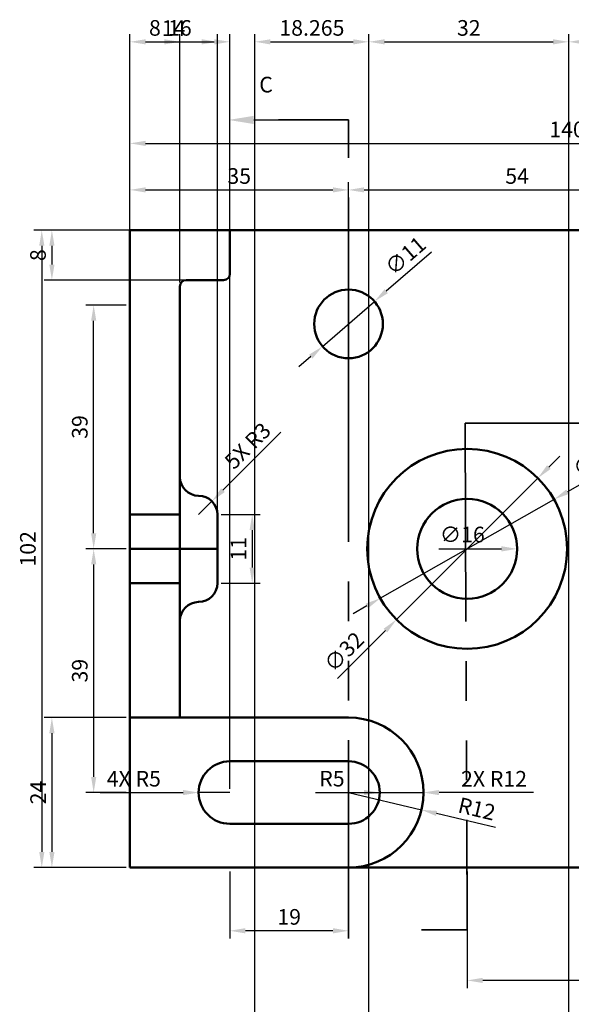
# Model space of a CAD drawing. Units: millimetres. Extents: x 2432 to 2611, y 2100 to 2357.
# Tile 2 of 3: x 2432 to 2521, y 2199 to 2357. Entities that reach past the tile are written whole.
import ezdxf
from ezdxf import colors
from ezdxf.entities.mleader import LeaderData, LeaderLine
from ezdxf.math import Vec2, Vec3

# ---------------------------------------------------------------- set-up
doc = ezdxf.new("R2010")
doc.units = ezdxf.units.MM
doc.linetypes.add('PHANTOM', pattern=[63.5, 31.75, -6.35, 6.35, -6.35, 6.35, -6.35])
for name, color, linetype, lineweight in [('M-DIMS', 2, 'Continuous', 25), ('M-OUTL', 7, 'Continuous', 50), ('M-SECT', 1, 'PHANTOM', 35), ('M-TEXT', 3, 'Continuous', 25)]:
    doc.layers.add(name, color=color, linetype=linetype, lineweight=lineweight)
doc.styles.get("Standard").update_dxf_attribs({"font": 'arial.ttf'})
doc.dimstyles.new('ISO-25', dxfattribs={"dimtxt": 2.5, "dimasz": 2.5, "dimexe": 1.25, "dimexo": 0.625, "dimtad": 1, "dimtxsty": 'Standard', "dimcen": 2.5, "dimadec": 0, "dimazin": 0, "dimtfac": 1, "dimtmove": 0, "dimatfit": 3, "dimfxl": 1, "dimarcsym": 0})

# ---------------------------------------------------------------- blocks, each defined once
blk = doc.blocks.new('*D1')
at = {"layer": 'Defpoints', "color": 0, "transparency": 16777216}
for p in [(2485.07, 2329.49), (2450.07, 2323.05), (2485.07, 2323.05)]:
    blk.add_point(p, dxfattribs=at)
at = {"layer": 'M-DIMS', "color": 0, "lineweight": -2, "transparency": 16777216}
for p, q in [((2450.07, 2323.67), (2450.07, 2330.74)), ((2485.07, 2323.67), (2485.07, 2330.74)), ((2452.57, 2329.49), (2482.57, 2329.49))]:
    blk.add_line(p, q, dxfattribs=at)
at = {"layer": 'M-DIMS', "color": 0, "transparency": 16777216}
for points in [[(2452.57, 2329.91), (2452.57, 2329.08), (2450.07, 2329.49)], [(2482.57, 2329.91), (2482.57, 2329.08), (2485.07, 2329.49)]]:
    blk.add_solid(points, dxfattribs=at)
at = {"layer": 'M-DIMS', "color": 0, "transparency": 16777216, "insert": (2467.57, 2331.39), "char_height": 2.5, "attachment_point": 5}
blk.add_mtext('35', dxfattribs=at)
blk = doc.blocks.new('*D2')
at = {"layer": 'Defpoints', "color": 0, "transparency": 16777216}
for p in [(2539.07, 2329.49), (2485.07, 2323.05), (2539.07, 2323.05)]:
    blk.add_point(p, dxfattribs=at)
at = {"layer": 'M-DIMS', "color": 0, "lineweight": -2, "transparency": 16777216}
for p, q in [((2485.07, 2323.67), (2485.07, 2330.74)), ((2539.07, 2323.67), (2539.07, 2330.74)), ((2487.57, 2329.49), (2536.57, 2329.49))]:
    blk.add_line(p, q, dxfattribs=at)
at = {"layer": 'M-DIMS', "color": 0, "transparency": 16777216}
for points in [[(2487.57, 2329.91), (2487.57, 2329.08), (2485.07, 2329.49)], [(2536.57, 2329.91), (2536.57, 2329.08), (2539.07, 2329.49)]]:
    blk.add_solid(points, dxfattribs=at)
at = {"layer": 'M-DIMS', "color": 0, "transparency": 16777216, "insert": (2512.07, 2331.39), "char_height": 2.5, "attachment_point": 5}
blk.add_mtext('54', dxfattribs=at)
blk = doc.blocks.new('*D3')
at = {"layer": 'Defpoints', "color": 0, "transparency": 16777216}
for p in [(2590.07, 2336.94), (2450.07, 2323.05), (2590.07, 2323.05)]:
    blk.add_point(p, dxfattribs=at)
at = {"layer": 'M-DIMS', "color": 0, "lineweight": -2, "transparency": 16777216}
for p, q in [((2450.07, 2323.67), (2450.07, 2338.19)), ((2452.57, 2336.94), (2587.57, 2336.94)), ((2590.07, 2323.67), (2590.07, 2338.19))]:
    blk.add_line(p, q, dxfattribs=at)
at = {"layer": 'M-DIMS', "color": 0, "transparency": 16777216}
for points in [[(2452.57, 2337.35), (2452.57, 2336.52), (2450.07, 2336.94)], [(2587.57, 2337.35), (2587.57, 2336.52), (2590.07, 2336.94)]]:
    blk.add_solid(points, dxfattribs=at)
at = {"layer": 'M-DIMS', "color": 0, "transparency": 16777216, "insert": (2520.07, 2338.84), "char_height": 2.5, "attachment_point": 5}
blk.add_mtext('140', dxfattribs=at)
blk = doc.blocks.new('*D9')
at = {"layer": 'Defpoints', "color": 0, "transparency": 16777216}
for p in [(2504.07, 2221.05), (2590.07, 2221.05), (2504.07, 2202.99)]:
    blk.add_point(p, dxfattribs=at)
at = {"layer": 'M-DIMS', "color": 0, "lineweight": -2, "transparency": 16777216}
for p, q in [((2504.07, 2220.42), (2504.07, 2201.74)), ((2590.07, 2220.42), (2590.07, 2201.74)), ((2587.57, 2202.99), (2506.57, 2202.99))]:
    blk.add_line(p, q, dxfattribs=at)
at = {"layer": 'M-DIMS', "color": 0, "transparency": 16777216}
for points in [[(2506.57, 2203.4), (2506.57, 2202.57), (2504.07, 2202.99)], [(2587.57, 2203.4), (2587.57, 2202.57), (2590.07, 2202.99)]]:
    blk.add_solid(points, dxfattribs=at)
at = {"layer": 'M-DIMS', "color": 0, "transparency": 16777216, "insert": (2547.07, 2204.89), "char_height": 2.5, "attachment_point": 5}
blk.add_mtext('86', dxfattribs=at)
blk = doc.blocks.new('*D10')
at = {"layer": 'Defpoints', "color": 0, "transparency": 16777216}
for p in [(2466.07, 2221.05), (2485.07, 2221.05), (2466.07, 2210.93)]:
    blk.add_point(p, dxfattribs=at)
at = {"layer": 'M-DIMS', "color": 0, "lineweight": -2, "transparency": 16777216}
for p, q in [((2466.07, 2220.42), (2466.07, 2209.68)), ((2485.07, 2220.42), (2485.07, 2209.68)), ((2482.57, 2210.93), (2468.57, 2210.93))]:
    blk.add_line(p, q, dxfattribs=at)
at = {"layer": 'M-DIMS', "color": 0, "transparency": 16777216}
for points in [[(2468.57, 2211.35), (2468.57, 2210.51), (2466.07, 2210.93)], [(2482.57, 2211.35), (2482.57, 2210.51), (2485.07, 2210.93)]]:
    blk.add_solid(points, dxfattribs=at)
at = {"layer": 'M-DIMS', "color": 0, "transparency": 16777216, "insert": (2475.57, 2212.83), "char_height": 2.5, "attachment_point": 5}
blk.add_mtext('19', dxfattribs=at)
blk = doc.blocks.new('*D11')
at = {"layer": 'Defpoints', "color": 0, "transparency": 16777216}
for p in [(2464.07, 2277.55), (2464.07, 2266.55), (2469.65, 2266.55)]:
    blk.add_point(p, dxfattribs=at)
at = {"layer": 'M-DIMS', "color": 0, "lineweight": -2, "transparency": 16777216}
for p, q in [((2464.7, 2277.55), (2470.9, 2277.55)), ((2469.65, 2275.05), (2469.65, 2269.05)), ((2464.7, 2266.55), (2470.9, 2266.55))]:
    blk.add_line(p, q, dxfattribs=at)
at = {"layer": 'M-DIMS', "color": 0, "transparency": 16777216}
for points in [[(2469.23, 2275.05), (2470.06, 2275.05), (2469.65, 2277.55)], [(2469.23, 2269.05), (2470.06, 2269.05), (2469.65, 2266.55)]]:
    blk.add_solid(points, dxfattribs=at)
at = {"layer": 'M-DIMS', "color": 0, "transparency": 16777216, "insert": (2467.77, 2272.05), "char_height": 2.5, "attachment_point": 5, "rotation": 90}
blk.add_mtext('11', dxfattribs=at)
blk = doc.blocks.new('*D12')
at = {"layer": 'Defpoints', "color": 0, "transparency": 16777216}
for p in [(2444.26, 2311.05), (2450.07, 2311.05), (2450.07, 2272.05)]:
    blk.add_point(p, dxfattribs=at)
at = {"layer": 'M-DIMS', "color": 0, "lineweight": -2, "transparency": 16777216}
for p, q in [((2449.45, 2311.05), (2443.01, 2311.05)), ((2444.26, 2274.55), (2444.26, 2308.55)), ((2449.45, 2272.05), (2443.01, 2272.05))]:
    blk.add_line(p, q, dxfattribs=at)
at = {"layer": 'M-DIMS', "color": 0, "transparency": 16777216}
for points in [[(2443.85, 2308.55), (2444.68, 2308.55), (2444.26, 2311.05)], [(2443.85, 2274.55), (2444.68, 2274.55), (2444.26, 2272.05)]]:
    blk.add_solid(points, dxfattribs=at)
at = {"layer": 'M-DIMS', "color": 0, "transparency": 16777216, "insert": (2442.36, 2291.55), "char_height": 2.5, "attachment_point": 5, "rotation": 90}
blk.add_mtext('39', dxfattribs=at)
blk = doc.blocks.new('*D13')
at = {"layer": 'Defpoints', "color": 0, "transparency": 16777216}
for p in [(2450.07, 2272.05), (2444.26, 2233.05), (2450.07, 2233.05)]:
    blk.add_point(p, dxfattribs=at)
at = {"layer": 'M-DIMS', "color": 0, "lineweight": -2, "transparency": 16777216}
for p, q in [((2449.45, 2272.05), (2443.01, 2272.05)), ((2444.26, 2269.55), (2444.26, 2235.55)), ((2449.45, 2233.05), (2443.01, 2233.05))]:
    blk.add_line(p, q, dxfattribs=at)
at = {"layer": 'M-DIMS', "color": 0, "transparency": 16777216}
for points in [[(2443.85, 2269.55), (2444.68, 2269.55), (2444.26, 2272.05)], [(2443.85, 2235.55), (2444.68, 2235.55), (2444.26, 2233.05)]]:
    blk.add_solid(points, dxfattribs=at)
at = {"layer": 'M-DIMS', "color": 0, "transparency": 16777216, "insert": (2442.36, 2252.55), "char_height": 2.5, "attachment_point": 5, "rotation": 90}
blk.add_mtext('39', dxfattribs=at)
blk = doc.blocks.new('*D14')
at = {"layer": 'Defpoints', "color": 0, "transparency": 16777216}
for p in [(2450.07, 2323.05), (2435.95, 2221.05), (2450.07, 2221.05)]:
    blk.add_point(p, dxfattribs=at)
at = {"layer": 'M-DIMS', "color": 0, "lineweight": -2, "transparency": 16777216}
for p, q in [((2449.45, 2323.05), (2434.7, 2323.05)), ((2435.95, 2320.55), (2435.95, 2223.55)), ((2449.45, 2221.05), (2434.7, 2221.05))]:
    blk.add_line(p, q, dxfattribs=at)
at = {"layer": 'M-DIMS', "color": 0, "transparency": 16777216}
for points in [[(2435.54, 2320.55), (2436.37, 2320.55), (2435.95, 2323.05)], [(2435.54, 2223.55), (2436.37, 2223.55), (2435.95, 2221.05)]]:
    blk.add_solid(points, dxfattribs=at)
at = {"layer": 'M-DIMS', "color": 0, "transparency": 16777216, "insert": (2434.05, 2272.05), "char_height": 2.5, "attachment_point": 5, "rotation": 90}
blk.add_mtext('102', dxfattribs=at)
blk = doc.blocks.new('*D15')
at = {"layer": 'Defpoints', "color": 0, "transparency": 16777216}
for p in [(2489.24, 2311.65), (2480.91, 2304.45)]:
    blk.add_point(p, dxfattribs=at)
at = {"layer": 'M-DIMS', "color": 0, "lineweight": -2, "transparency": 16777216}
for p, q in [((2498.36, 2319.54), (2491.13, 2313.28)), ((2480.91, 2304.45), (2489.24, 2311.65)), ((2479.02, 2302.82), (2477.13, 2301.18))]:
    blk.add_line(p, q, dxfattribs=at)
at = {"layer": 'M-DIMS', "color": 0, "transparency": 16777216}
for points in [[(2490.85, 2313.6), (2491.4, 2312.97), (2489.24, 2311.65)], [(2478.75, 2303.13), (2479.3, 2302.5), (2480.91, 2304.45)]]:
    blk.add_solid(points, dxfattribs=at)
at = {"layer": 'M-DIMS', "color": 0, "transparency": 16777216, "insert": (2494.4, 2318.72), "char_height": 2.5, "attachment_point": 5, "rotation": 40.8461}
blk.add_mtext('∅11', dxfattribs=at)
blk = doc.blocks.new('*D19')
at = {"layer": 'Defpoints', "color": 0, "transparency": 16777216}
for p in [(2496.07, 2272.05), (2512.07, 2272.05)]:
    blk.add_point(p, dxfattribs=at)
at = {"layer": 'M-DIMS', "color": 0, "lineweight": -2, "transparency": 16777216}
blk.add_line((2499.53, 2272.05), (2509.57, 2272.05), dxfattribs=at)
at = {"layer": 'M-DIMS', "color": 0, "transparency": 16777216}
blk.add_solid([(2509.57, 2272.47), (2509.57, 2271.63), (2512.07, 2272.05)], dxfattribs=at)
at = {"layer": 'M-DIMS', "color": 0, "transparency": 16777216, "insert": (2503.3, 2274.02), "char_height": 2.5, "attachment_point": 5}
blk.add_mtext('∅16', dxfattribs=at)
blk = doc.blocks.new('*D20')
at = {"layer": 'Defpoints', "color": 0, "transparency": 16777216}
for p in [(2517.98, 2279.96), (2490.16, 2264.14)]:
    blk.add_point(p, dxfattribs=at)
at = {"layer": 'M-DIMS', "color": 0, "lineweight": -2, "transparency": 16777216}
for p, q in [((2528.87, 2286.15), (2520.16, 2281.19)), ((2490.16, 2264.14), (2517.98, 2279.96)), ((2487.99, 2262.91), (2485.82, 2261.67))]:
    blk.add_line(p, q, dxfattribs=at)
at = {"layer": 'M-DIMS', "color": 0, "transparency": 16777216}
for points in [[(2519.95, 2281.55), (2520.36, 2280.83), (2517.98, 2279.96)], [(2487.79, 2263.27), (2488.2, 2262.54), (2490.16, 2264.14)]]:
    blk.add_solid(points, dxfattribs=at)
at = {"layer": 'M-DIMS', "color": 0, "transparency": 16777216, "insert": (2524.63, 2286), "char_height": 2.5, "attachment_point": 5, "rotation": 29.6157}
blk.add_mtext('∅32', dxfattribs=at)
blk = doc.blocks.new('*D21')
at = {"layer": 'Defpoints', "color": 0, "transparency": 16777216}
for p in [(2485.07, 2233.05), (2490.07, 2233.05)]:
    blk.add_point(p, dxfattribs=at)
at = {"layer": 'M-DIMS', "color": 0, "lineweight": -2, "transparency": 16777216}
blk.add_line((2479.77, 2233.05), (2487.57, 2233.05), dxfattribs=at)
at = {"layer": 'M-DIMS', "color": 0, "transparency": 16777216}
blk.add_solid([(2487.57, 2233.47), (2487.57, 2232.63), (2490.07, 2233.05)], dxfattribs=at)
at = {"layer": 'M-DIMS', "color": 0, "transparency": 16777216, "insert": (2482.42, 2234.95), "char_height": 2.5, "attachment_point": 5}
blk.add_mtext('R5', dxfattribs=at)
blk = doc.blocks.new('*D22')
at = {"layer": 'Defpoints', "color": 0, "transparency": 16777216}
for p in [(2485.07, 2233.05), (2496.75, 2230.28)]:
    blk.add_point(p, dxfattribs=at)
at = {"layer": 'M-DIMS', "color": 0, "lineweight": -2, "transparency": 16777216}
for p, q in [((2485.07, 2233.05), (2496.75, 2230.28)), ((2508.62, 2227.47), (2499.18, 2229.7))]:
    blk.add_line(p, q, dxfattribs=at)
at = {"layer": 'M-DIMS', "color": 0, "transparency": 16777216}
blk.add_solid([(2499.28, 2230.11), (2499.09, 2229.3), (2496.75, 2230.28)], dxfattribs=at)
at = {"layer": 'M-DIMS', "color": 0, "transparency": 16777216, "insert": (2505.55, 2230.13), "char_height": 2.5, "attachment_point": 5, "rotation": 346.6592}
blk.add_mtext('R12', dxfattribs=at)
blk = doc.blocks.new('*D34')
at = {"layer": 'Defpoints', "color": 0, "transparency": 16777216}
for p in [(2458.07, 2353.19), (2450.07, 2323.05), (2458.07, 2314.05)]:
    blk.add_point(p, dxfattribs=at)
at = {"layer": 'M-DIMS', "color": 0, "lineweight": -2, "transparency": 16777216}
for p, q in [((2450.07, 2323.67), (2450.07, 2354.44)), ((2458.07, 2314.67), (2458.07, 2354.44)), ((2452.57, 2353.19), (2455.57, 2353.19))]:
    blk.add_line(p, q, dxfattribs=at)
at = {"layer": 'M-DIMS', "color": 0, "transparency": 16777216}
for points in [[(2452.57, 2353.6), (2452.57, 2352.77), (2450.07, 2353.19)], [(2455.57, 2353.6), (2455.57, 2352.77), (2458.07, 2353.19)]]:
    blk.add_solid(points, dxfattribs=at)
at = {"layer": 'M-DIMS', "color": 0, "transparency": 16777216, "insert": (2454.07, 2355.09), "char_height": 2.5, "attachment_point": 5}
blk.add_mtext('8', dxfattribs=at)
blk = doc.blocks.new('*D35')
at = {"layer": 'Defpoints', "color": 0, "transparency": 16777216}
for p in [(2466.07, 2353.19), (2450.07, 2323.05), (2466.07, 2323.05)]:
    blk.add_point(p, dxfattribs=at)
at = {"layer": 'M-DIMS', "color": 0, "lineweight": -2, "transparency": 16777216}
for p, q in [((2450.07, 2323.67), (2450.07, 2354.44)), ((2466.07, 2323.67), (2466.07, 2354.44)), ((2452.57, 2353.19), (2463.57, 2353.19))]:
    blk.add_line(p, q, dxfattribs=at)
at = {"layer": 'M-DIMS', "color": 0, "transparency": 16777216}
for points in [[(2452.57, 2353.6), (2452.57, 2352.77), (2450.07, 2353.19)], [(2463.57, 2353.6), (2463.57, 2352.77), (2466.07, 2353.19)]]:
    blk.add_solid(points, dxfattribs=at)
at = {"layer": 'M-DIMS', "color": 0, "transparency": 16777216, "insert": (2458.07, 2355.09), "char_height": 2.5, "attachment_point": 5}
blk.add_mtext('16', dxfattribs=at)
blk = doc.blocks.new('*D36')
at = {"layer": 'Defpoints', "color": 0, "transparency": 16777216}
for p in [(2466.07, 2323.05), (2437.57, 2315.05), (2462.67, 2315.05)]:
    blk.add_point(p, dxfattribs=at)
at = {"layer": 'M-DIMS', "color": 0, "lineweight": -2, "transparency": 16777216}
for p, q in [((2465.45, 2323.05), (2436.32, 2323.05)), ((2437.57, 2320.55), (2437.57, 2317.55)), ((2462.05, 2315.05), (2436.32, 2315.05))]:
    blk.add_line(p, q, dxfattribs=at)
at = {"layer": 'M-DIMS', "color": 0, "transparency": 16777216}
for points in [[(2437.16, 2320.55), (2437.99, 2320.55), (2437.57, 2323.05)], [(2437.16, 2317.55), (2437.99, 2317.55), (2437.57, 2315.05)]]:
    blk.add_solid(points, dxfattribs=at)
at = {"layer": 'M-DIMS', "color": 0, "transparency": 16777216, "insert": (2435.67, 2319.05), "char_height": 2.5, "attachment_point": 5, "rotation": 90}
blk.add_mtext('8', dxfattribs=at)
blk = doc.blocks.new('*D40')
at = {"layer": 'Defpoints', "color": 0, "transparency": 16777216}
for p in [(2450.07, 2245.05), (2437.57, 2221.05), (2450.07, 2221.05)]:
    blk.add_point(p, dxfattribs=at)
at = {"layer": 'M-DIMS', "color": 0, "lineweight": -2, "transparency": 16777216}
for p, q in [((2449.45, 2245.05), (2436.32, 2245.05)), ((2437.57, 2242.55), (2437.57, 2223.55)), ((2449.45, 2221.05), (2436.32, 2221.05))]:
    blk.add_line(p, q, dxfattribs=at)
at = {"layer": 'M-DIMS', "color": 0, "transparency": 16777216}
for points in [[(2437.16, 2242.55), (2437.99, 2242.55), (2437.57, 2245.05)], [(2437.16, 2223.55), (2437.99, 2223.55), (2437.57, 2221.05)]]:
    blk.add_solid(points, dxfattribs=at)
at = {"layer": 'M-DIMS', "color": 0, "transparency": 16777216, "insert": (2435.69, 2233.05), "char_height": 2.5, "attachment_point": 5, "rotation": 90}
blk.add_mtext('24', dxfattribs=at)
blk = doc.blocks.new('*D41')
at = {"layer": 'Defpoints', "color": 0, "transparency": 16777216}
for p in [(2466.07, 2353.19), (2466.07, 2233.05), (2450.07, 2221.05)]:
    blk.add_point(p, dxfattribs=at)
at = {"layer": 'M-DIMS', "color": 0, "lineweight": -2, "transparency": 16777216}
for p, q in [((2450.07, 2221.67), (2450.07, 2354.44)), ((2466.07, 2233.67), (2466.07, 2354.44)), ((2452.57, 2353.19), (2463.57, 2353.19))]:
    blk.add_line(p, q, dxfattribs=at)
at = {"layer": 'M-DIMS', "color": 0, "transparency": 16777216}
for points in [[(2452.57, 2353.6), (2452.57, 2352.77), (2450.07, 2353.19)], [(2463.57, 2353.6), (2463.57, 2352.77), (2466.07, 2353.19)]]:
    blk.add_solid(points, dxfattribs=at)
at = {"layer": 'M-DIMS', "color": 0, "transparency": 16777216, "insert": (2458.07, 2355.09), "char_height": 2.5, "attachment_point": 5}
blk.add_mtext('16', dxfattribs=at)
blk = doc.blocks.new('*D42')
at = {"layer": 'Defpoints', "color": 0, "transparency": 16777216}
for p in [(2464.07, 2353.19), (2450.07, 2277.55), (2464.07, 2272.05)]:
    blk.add_point(p, dxfattribs=at)
at = {"layer": 'M-DIMS', "color": 0, "lineweight": -2, "transparency": 16777216}
for p, q in [((2450.07, 2278.17), (2450.07, 2354.44)), ((2464.07, 2272.67), (2464.07, 2354.44)), ((2452.57, 2353.19), (2461.57, 2353.19))]:
    blk.add_line(p, q, dxfattribs=at)
at = {"layer": 'M-DIMS', "color": 0, "transparency": 16777216}
for points in [[(2452.57, 2353.6), (2452.57, 2352.77), (2450.07, 2353.19)], [(2461.57, 2353.6), (2461.57, 2352.77), (2464.07, 2353.19)]]:
    blk.add_solid(points, dxfattribs=at)
at = {"layer": 'M-DIMS', "color": 0, "transparency": 16777216, "insert": (2457.07, 2355.07), "char_height": 2.5, "attachment_point": 5}
blk.add_mtext('14', dxfattribs=at)
blk = doc.blocks.new('*D43')
at = {"layer": 'Defpoints', "color": 0, "transparency": 16777216}
for p in [(2488.34, 2353.19), (2470.07, 2151.26), (2488.34, 2145.26)]:
    blk.add_point(p, dxfattribs=at)
at = {"layer": 'M-DIMS', "color": 0, "lineweight": -2, "transparency": 16777216}
for p, q in [((2470.07, 2151.89), (2470.07, 2354.44)), ((2488.34, 2145.89), (2488.34, 2354.44)), ((2472.57, 2353.19), (2485.84, 2353.19))]:
    blk.add_line(p, q, dxfattribs=at)
at = {"layer": 'M-DIMS', "color": 0, "transparency": 16777216}
for points in [[(2472.57, 2353.6), (2472.57, 2352.77), (2470.07, 2353.19)], [(2485.84, 2353.6), (2485.84, 2352.77), (2488.34, 2353.19)]]:
    blk.add_solid(points, dxfattribs=at)
at = {"layer": 'M-DIMS', "color": 0, "transparency": 16777216, "insert": (2479.21, 2355.09), "char_height": 2.5, "attachment_point": 5}
blk.add_mtext('18.265', dxfattribs=at)
blk = doc.blocks.new('*D44')
at = {"layer": 'Defpoints', "color": 0, "transparency": 16777216}
for p in [(2520.34, 2353.19), (2488.34, 2145.26), (2520.34, 2145.26)]:
    blk.add_point(p, dxfattribs=at)
at = {"layer": 'M-DIMS', "color": 0, "lineweight": -2, "transparency": 16777216}
for p, q in [((2488.34, 2145.89), (2488.34, 2354.44)), ((2520.34, 2145.89), (2520.34, 2354.44)), ((2490.84, 2353.19), (2517.84, 2353.19))]:
    blk.add_line(p, q, dxfattribs=at)
at = {"layer": 'M-DIMS', "color": 0, "transparency": 16777216}
for points in [[(2490.84, 2353.6), (2490.84, 2352.77), (2488.34, 2353.19)], [(2517.84, 2353.6), (2517.84, 2352.77), (2520.34, 2353.19)]]:
    blk.add_solid(points, dxfattribs=at)
at = {"layer": 'M-DIMS', "color": 0, "transparency": 16777216, "insert": (2504.34, 2355.09), "char_height": 2.5, "attachment_point": 5}
blk.add_mtext('32', dxfattribs=at)
blk = doc.blocks.new('*D45')
at = {"layer": 'Defpoints', "color": 0, "transparency": 16777216}
for p in [(2534.07, 2353.19), (2534.07, 2151.26), (2520.34, 2145.26)]:
    blk.add_point(p, dxfattribs=at)
at = {"layer": 'M-DIMS', "color": 0, "lineweight": -2, "transparency": 16777216}
for p, q in [((2520.34, 2145.89), (2520.34, 2354.44)), ((2534.07, 2151.89), (2534.07, 2354.44)), ((2522.84, 2353.19), (2531.57, 2353.19))]:
    blk.add_line(p, q, dxfattribs=at)
at = {"layer": 'M-DIMS', "color": 0, "transparency": 16777216}
for points in [[(2522.84, 2353.6), (2522.84, 2352.77), (2520.34, 2353.19)], [(2531.57, 2353.6), (2531.57, 2352.77), (2534.07, 2353.19)]]:
    blk.add_solid(points, dxfattribs=at)
at = {"layer": 'M-DIMS', "color": 0, "transparency": 16777216, "insert": (2527.21, 2355.09), "char_height": 2.5, "attachment_point": 5}
blk.add_mtext('13.735', dxfattribs=at)
blk = doc.blocks.new('*D51')
at = {"layer": 'Defpoints', "color": 0, "transparency": 16777216}
for p in [(2515.39, 2283.36), (2492.76, 2260.74)]:
    blk.add_point(p, dxfattribs=at)
at = {"layer": 'M-DIMS', "color": 0, "lineweight": -2, "transparency": 16777216}
for p, q in [((2517.16, 2285.13), (2518.93, 2286.9)), ((2515.39, 2283.36), (2492.76, 2260.74)), ((2483.31, 2251.29), (2490.99, 2258.97))]:
    blk.add_line(p, q, dxfattribs=at)
at = {"layer": 'M-DIMS', "color": 0, "transparency": 16777216}
for points in [[(2516.86, 2285.42), (2517.45, 2284.83), (2515.39, 2283.36)], [(2490.7, 2259.27), (2491.28, 2258.68), (2492.76, 2260.74)]]:
    blk.add_solid(points, dxfattribs=at)
at = {"layer": 'M-DIMS', "color": 0, "transparency": 16777216, "insert": (2484.57, 2255.35), "char_height": 2.5, "attachment_point": 5, "rotation": 44.9868}
blk.add_mtext('∅32', dxfattribs=at)
blk = doc.blocks.new('*D52')
at = {"layer": 'Defpoints', "color": 0, "transparency": 16777216}
for p in [(2485.07, 2233.05), (2497.07, 2233.05)]:
    blk.add_point(p, dxfattribs=at)
at = {"layer": 'M-DIMS', "color": 0, "lineweight": -2, "transparency": 16777216}
for p, q in [((2485.07, 2233.05), (2497.07, 2233.05)), ((2514.69, 2233.05), (2499.57, 2233.05))]:
    blk.add_line(p, q, dxfattribs=at)
at = {"layer": 'M-DIMS', "color": 0, "transparency": 16777216}
blk.add_solid([(2499.57, 2233.47), (2499.57, 2232.63), (2497.07, 2233.05)], dxfattribs=at)
at = {"layer": 'M-DIMS', "color": 0, "transparency": 16777216, "insert": (2508.38, 2234.93), "char_height": 2.5, "attachment_point": 5, "rotation": 359.9985}
blk.add_mtext('2X R12', dxfattribs=at)
blk = doc.blocks.new('*D53')
at = {"layer": 'Defpoints', "color": 0, "transparency": 16777216}
for p in [(2461.07, 2233.05), (2466.07, 2233.05)]:
    blk.add_point(p, dxfattribs=at)
at = {"layer": 'M-DIMS', "color": 0, "lineweight": -2, "transparency": 16777216}
for p, q in [((2445.3, 2233.05), (2458.57, 2233.05)), ((2466.07, 2233.05), (2461.07, 2233.05))]:
    blk.add_line(p, q, dxfattribs=at)
at = {"layer": 'M-DIMS', "color": 0, "transparency": 16777216}
blk.add_solid([(2458.57, 2233.47), (2458.57, 2232.63), (2461.07, 2233.05)], dxfattribs=at)
at = {"layer": 'M-DIMS', "color": 0, "transparency": 16777216, "insert": (2450.69, 2234.94), "char_height": 2.5, "attachment_point": 5, "rotation": 0.0036}
blk.add_mtext('4X R5', dxfattribs=at)
blk = doc.blocks.new('*D55')
at = {"layer": 'Defpoints', "color": 0, "transparency": 16777216}
for p in [(2463.2, 2279.67), (2461.07, 2277.55)]:
    blk.add_point(p, dxfattribs=at)
at = {"layer": 'M-DIMS', "color": 0, "lineweight": -2, "transparency": 16777216}
for p, q in [((2474.26, 2290.74), (2464.96, 2281.44)), ((2461.07, 2277.55), (2463.2, 2279.67))]:
    blk.add_line(p, q, dxfattribs=at)
at = {"layer": 'M-DIMS', "color": 0, "transparency": 16777216}
blk.add_solid([(2464.67, 2281.73), (2465.26, 2281.14), (2463.2, 2279.67)], dxfattribs=at)
at = {"layer": 'M-DIMS', "color": 0, "transparency": 16777216, "insert": (2469.15, 2288.32), "char_height": 2.5, "attachment_point": 5, "rotation": 45.0031}
blk.add_mtext('5X R3', dxfattribs=at)

msp = doc.modelspace()

# ---------------------------------------------------------------- linework, layer by layer
at = {"layer": 'M-OUTL'}
for p, q in [((2450.0745, 2323.0493), (2590.0745, 2323.0493)), ((2450.0745, 2221.0493), (2450.0745, 2323.0493)), ((2450.0745, 2323.0493), (2485.0745, 2323.0493)), ((2485.0745, 2323.0493), (2466.0745, 2323.0493)), ((2466.0745, 2316.0493), (2466.0745, 2323.0493)), ((2459.2745, 2315.0493), (2459.0745, 2315.0493)), ((2462.6745, 2315.0493), (2459.2745, 2315.0493)), ((2465.0745, 2315.0493), (2462.6745, 2315.0493)), ((2458.0745, 2314.0493), (2458.0745, 2245.0493)), ((2458.0745, 2277.5493), (2458.0745, 2280.5493)), ((2458.0745, 2277.5493), (2450.0745, 2277.5493)), ((2464.0745, 2272.0493), (2464.0745, 2277.5493)), ((2464.0745, 2277.5493), (2464.0745, 2272.0493)), ((2450.0745, 2272.0493), (2464.0745, 2272.0493)), ((2464.0745, 2272.0493), (2464.0745, 2266.5493)), ((2458.0745, 2266.5493), (2450.0745, 2266.5493)), ((2458.0745, 2266.5493), (2458.0745, 2263.5493)), ((2485.0745, 2245.0493), (2450.0745, 2245.0493)), ((2466.0745, 2238.0493), (2485.0745, 2238.0493)), ((2466.0745, 2228.0493), (2485.0745, 2228.0493)), ((2590.0745, 2221.0493), (2450.0745, 2221.0493))]:
    msp.add_line(p, q, dxfattribs=at)
for centre, radius in [((2485.0745, 2308.0493), 5.5), ((2504.0745, 2272.0493), 16), ((2504.0745, 2272.0493), 8)]:
    msp.add_circle(centre, radius, dxfattribs=at)
for centre, radius, start, end in [((2459.0745, 2314.0493), 1, 90, 180), ((2465.0745, 2316.0493), 1, 270, 0), ((2461.0745, 2283.5493), 3, 180, 270), ((2461.0745, 2277.5493), 3, 0, 90), ((2461.0745, 2266.5493), 3, 270, 0), ((2461.0745, 2260.5493), 3, 90, 180), ((2485.0745, 2233.0493), 12, 270, 90), ((2466.0745, 2233.0493), 5, 90, 270), ((2485.0745, 2233.0493), 5, 270, 90)]:
    msp.add_arc(centre, radius, start, end, dxfattribs=at)
at = {"layer": 'M-SECT'}
for p, q in [((2485.0745, 2340.6874), (2473.885, 2340.6874)), ((2485.0745, 2296.5285), (2485.0745, 2340.6874)), ((2485.0745, 2209.6812), (2485.0745, 2296.5285)), ((2511.6649, 2292.1705), (2503.7481, 2292.1705)), ((2503.7481, 2292.1705), (2504.0745, 2211.0799)), ((2539.0745, 2292.1705), (2511.6649, 2292.1705)), ((2485.0745, 2233.0493), (2485.0745, 2209.6812)), ((2504.0745, 2211.0799), (2496.7749, 2211.0799))]:
    msp.add_line(p, q, dxfattribs=at)

# ---------------------------------------------------------------- texts
at = {"layer": 'M-TEXT', "insert": (2470.7803, 2347.5928), "char_height": 2.5, "attachment_point": 1}
msp.add_mtext_dynamic_manual_height_columns('C', width=14.294214, gutter_width=12.5, heights=[0], dxfattribs=at)

# ---------------------------------------------------------------- dimensions: what is measured, and where the dimension line sits
at = {"layer": 'M-DIMS'}
for base, p1, p2, override, picture, middle in [((2458.0745, 2353.1874), (2450.0745, 2323.0493), (2458.0745, 2314.0493), {"dimdec": 0, "dimlfac": 1, "dimrnd": 0, "dimzin": 0, "dimdsep": 46, "dimlunit": 2}, '*D34', (2454.0745, 2355.0889)), ((2466.0745, 2353.1874), (2450.0745, 2323.0493), (2466.0745, 2323.0493), {"dimdec": 0, "dimlfac": 1, "dimrnd": 0, "dimzin": 0, "dimdsep": 46, "dimlunit": 2}, '*D35', (2458.0745, 2355.0889)), ((2466.0745, 2353.1874), (2450.0745, 2221.0493), (2466.0745, 2233.0493), {"dimdec": 0, "dimlfac": 1, "dimrnd": 0, "dimzin": 0, "dimdsep": 46, "dimlunit": 2}, '*D41', (2458.0745, 2355.0889)), ((2464.0745, 2353.1874), (2450.0745, 2277.5493), (2464.0745, 2272.0493), {"dimdec": 0, "dimlfac": 1, "dimrnd": 0, "dimzin": 0, "dimdsep": 46, "dimlunit": 2}, '*D42', (2457.0745, 2355.0676)), ((2488.3395, 2353.1874), (2470.0745, 2151.2616), (2488.3395, 2145.2616), {"dimdec": 3, "dimlfac": 1, "dimrnd": 0, "dimzin": 0, "dimdsep": 46, "dimlunit": 2}, '*D43', (2479.207, 2355.0889)), ((2520.3395, 2353.1874), (2488.3395, 2145.2616), (2520.3395, 2145.2616), {"dimdec": 0, "dimlfac": 1, "dimrnd": 0, "dimzin": 0, "dimdsep": 46, "dimlunit": 2}, '*D44', (2504.3395, 2355.0897)), ((2534.0745, 2353.1874), (2520.3395, 2145.2616), (2534.0745, 2151.2616), {"dimdec": 3, "dimlfac": 1, "dimrnd": 0, "dimzin": 0, "dimdsep": 46, "dimlunit": 2}, '*D45', (2527.207, 2355.0897)), ((2590.0745, 2336.9374), (2450.0745, 2323.0493), (2590.0745, 2323.0493), {"dimclrd": 0, "dimclre": 0, "dimclrt": 0}, '*D3', (2520.0745, 2338.8389)), ((2485.0745, 2329.4923), (2450.0745, 2323.0493), (2485.0745, 2323.0493), {"dimclrd": 0, "dimclre": 0, "dimclrt": 0}, '*D1', (2467.5745, 2331.3946)), ((2539.0745, 2329.4923), (2485.0745, 2323.0493), (2539.0745, 2323.0493), {"dimclrd": 0, "dimclre": 0, "dimclrt": 0}, '*D2', (2512.0745, 2331.3886)), ((2466.0745, 2210.9312), (2485.0745, 2221.0493), (2466.0745, 2221.0493), {"dimclrd": 0, "dimclre": 0, "dimclrt": 0}, '*D10', (2475.5745, 2212.8326)), ((2504.0745, 2202.9855), (2590.0745, 2221.0493), (2504.0745, 2221.0493), {"dimclrd": 0, "dimclre": 0, "dimclrt": 0}, '*D9', (2547.0745, 2204.8869))]:
    dim = msp.add_linear_dim(base=base, p1=p1, p2=p2, dimstyle='ISO-25', override=override, dxfattribs=at)
    dim.commit()
    dim.dimension.update_dxf_attribs({"geometry": picture, "text_midpoint": middle})
for base, p1, p2, override, picture, middle in [((2435.9543, 2221.0493), (2450.0745, 2323.0493), (2450.0745, 2221.0493), {"dimclrd": 0, "dimclre": 0, "dimclrt": 0}, '*D14', (2434.0529, 2272.0493)), ((2437.5745, 2315.0493), (2466.0745, 2323.0493), (2462.6745, 2315.0493), {"dimdec": 0, "dimlfac": 1, "dimrnd": 0, "dimzin": 0, "dimdsep": 46, "dimlunit": 2}, '*D36', (2435.6731, 2319.0493)), ((2444.2624, 2311.0493), (2450.0745, 2272.0493), (2450.0745, 2311.0493), {"dimclrd": 0, "dimclre": 0, "dimclrt": 0}, '*D12', (2442.3601, 2291.5493)), ((2469.6483, 2266.5493), (2464.0745, 2277.5493), (2464.0745, 2266.5493), {"dimclrd": 0, "dimclre": 0, "dimclrt": 0}, '*D11', (2467.7681, 2272.0493)), ((2444.2624, 2233.0493), (2450.0745, 2272.0493), (2450.0745, 2233.0493), {"dimclrd": 0, "dimclre": 0, "dimclrt": 0}, '*D13', (2442.3601, 2252.5493)), ((2437.5745, 2221.0493), (2450.0745, 2245.0493), (2450.0745, 2221.0493), {"dimdec": 0, "dimlfac": 1, "dimrnd": 0, "dimzin": 0, "dimdsep": 46, "dimlunit": 2}, '*D40', (2435.6944, 2233.0493))]:
    dim = msp.add_linear_dim(base=base, p1=p1, p2=p2, angle=90, dimstyle='ISO-25', override=override, dxfattribs=at)
    dim.commit()
    dim.dimension.update_dxf_attribs({"geometry": picture, "text_midpoint": middle})
for p1, p2, picture, middle in [((2480.914, 2304.4522), (2489.2351, 2311.6465), '*D15', (2494.4017, 2318.7194)), ((2490.1648, 2264.1424), (2517.9843, 2279.9562), '*D20', (2524.6281, 2286.0004))]:
    dim = msp.add_diameter_dim_2p(p1=p1, p2=p2, dimstyle='ISO-25', override={"dimclrd": 0, "dimclre": 0, "dimclrt": 0}, dxfattribs=at)
    dim.commit()
    dim.dimension.update_dxf_attribs({"geometry": picture, "text_midpoint": middle})
for center, mpoint, text, picture, middle in [((2461.0745, 2277.5493), (2463.1958, 2279.6708), '5X <>', '*D55', (2469.1522, 2288.3182)), ((2466.0745, 2233.0493), (2461.0745, 2233.049), '4X <>', '*D53', (2450.6882, 2234.9447)), ((2485.0745, 2233.0493), (2497.0745, 2233.049), '2X <>', '*D52', (2508.3809, 2234.9297))]:
    dim = msp.add_radius_dim(center=center, mpoint=mpoint, text=text, dimstyle='ISO-25', override={"dimdec": 0, "dimlfac": 1, "dimrnd": 0, "dimzin": 0, "dimdsep": 46, "dimlunit": 2}, dxfattribs=at)
    dim.commit()
    dim.dimension.update_dxf_attribs({"geometry": picture, "text_midpoint": middle})
for p1, p2, override, picture, middle in [((2515.3909, 2283.3604), (2492.7582, 2260.7382), {"dimdec": 0, "dimlfac": 1, "dimrnd": 0, "dimzin": 0, "dimdsep": 46, "dimlunit": 2}, '*D51', (2485.9684, 2253.9516)), ((2496.0745, 2272.0493), (2512.0745, 2272.0493), {"dimclrd": 0, "dimclre": 0, "dimclrt": 0}, '*D19', (2503.2998, 2272.0493))]:
    dim = msp.add_diameter_dim_2p(p1=p1, p2=p2, dimstyle='ISO-25', override=override, dxfattribs=at)
    dim.commit()
    dim.dimension.update_dxf_attribs({"geometry": picture, "text_midpoint": middle, "dimtype": 163})
dim = msp.add_radius_dim(center=(2485.0745, 2233.0493), mpoint=(2490.0745, 2233.0493), dimstyle='ISO-25', override={"dimclrd": 0, "dimclre": 0, "dimclrt": 0}, dxfattribs=at)
dim.commit()
dim.dimension.update_dxf_attribs({"geometry": '*D21', "text_midpoint": (2482.4245, 2233.0493), "dimtype": 164})
dim = msp.add_radius_dim(center=(2485.0745, 2233.0493), mpoint=(2496.7507, 2230.2804), dimstyle='ISO-25', override={"dimclrd": 0, "dimclre": 0, "dimclrt": 0}, dxfattribs=at)
dim.commit()
dim.dimension.update_dxf_attribs({"geometry": '*D22', "text_midpoint": (2505.5516, 2230.1256)})

# ---------------------------------------------------------------- leaders
at = {"layer": 'M-TEXT'}
ml = msp.add_multileader_mtext('Standard', dxfattribs=at)
ml.set_content('', color=256)
ml.set_leader_properties()
ml.build(insert=Vec2(0, 0))
ctx = ml.context
ctx.base_point, ctx.plane_origin = Vec3(2485.0745, 2340.6874), Vec3(2465.885, 2340.6874)
notes = []
notes.append((ctx, [(0, (1, 1, 0), (2477.0745, 2340.6874), (1, 0), 8, [(0, [(2465.885, 2340.6874)], 0, [])])]))
ctx.mtext.insert, ctx.mtext.flow_direction = Vec3(2487.0745, 2342.6874), 5
for ctx, leaders in notes:
    for number, flags, end, landing, length, lines in leaders:
        leader = LeaderData()
        leader.index, (leader.has_last_leader_line, leader.has_dogleg_vector, leader.attachment_direction) = number, flags
        leader.last_leader_point, leader.dogleg_vector, leader.dogleg_length = Vec3(end), Vec3(landing), length
        for number, points, colour, breaks in lines:
            line = LeaderLine()
            line.index, line.vertices, line.color, line.breaks = number, Vec3.list(points), colors.encode_raw_color(colour), breaks
            leader.lines.append(line)
        ctx.leaders.append(leader)

doc.saveas('drawing.dxf')
